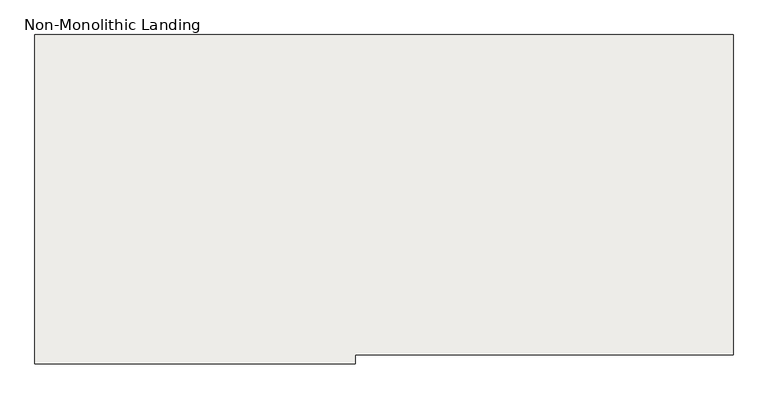
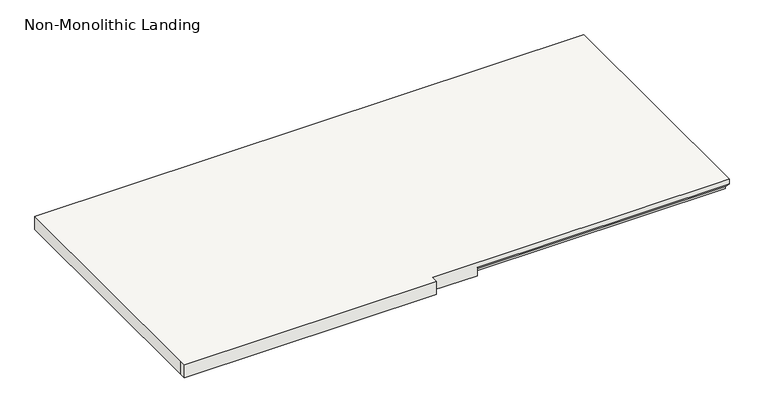
"""IFC4 building model written with IfcOpenShell, lengths in millimetres: slab geometry, Non-Monolithic Landing."""

from ifc_helpers import new_model, si_unit, origin, place, context, project, spatial, faceted_brep, source, transform, mapped, element, save


def non_monolithic_landing_8dc99a10(model_context):
    return source(origin(), model_context, "Body", "Brep", [
        faceted_brep([(-5380.4481169, -1269.3249317, 1919.8166667), (-5380.4481169, -1294.7249317, 1945.2166667), (-6294.8481169, -1294.7249317, 1945.2166667), (-6294.8481169, -1269.3249317, 1919.8166667), (-5380.4481169, -380.3249317, 1964.2666667), (-7372.0431792, -380.3249317, 1964.2666667), (-7372.0431792, -1294.7249317, 1964.2666667), (-7372.0431792, -1320.1249317, 1964.2666667), (-6457.6431792, -1320.1249317, 1964.2666667), (-6457.6431792, -1294.7249317, 1964.2666667), (-5380.4481169, -1294.7249317, 1964.2666667), (-6294.8481169, -1269.3249317, 1913.4666667), (-6294.8481169, -1294.7249317, 1913.4666667), (-6457.6431792, -1294.7249317, 1913.4666667), (-6457.6431792, -1320.1249317, 1913.4666667), (-7372.0431792, -1320.1249317, 1913.4666667), (-7372.0431792, -1294.7249317, 1913.4666667), (-7372.0431792, -380.3249317, 1913.4666667), (-5380.4481169, -380.3249317, 1913.4666667), (-5380.4481169, -1269.3249317, 1913.4666667)], [[[0, 1, 2, 3]], [[4, 5, 6, 7, 8, 9, 10]], [[11, 12, 13, 14, 15, 16, 17, 18, 19]], [[12, 11, 3, 2]], [[11, 19, 0, 3]], [[4, 10, 1, 0, 19, 18]], [[5, 4, 18, 17]], [[6, 5, 17, 16]], [[7, 6, 16, 15]], [[8, 7, 15, 14]], [[9, 8, 14, 13]], [[10, 9, 13, 12, 2, 1]]]),
    ])


if __name__ == "__main__":
    model = new_model("IFC4")
    model_context = context("Model", 3, world=origin())
    ifc_project = project(units=[si_unit("LENGTHUNIT", "METRE", prefix="MILLI")], contexts=[model_context])
    site = spatial("IfcSite", under=ifc_project)
    building = spatial("IfcBuilding", under=site)
    placement = place(None, origin())
    non_monolithic_landing_shape = non_monolithic_landing_8dc99a10(model_context)
    element("IfcSlab", 1, ObjectType="Non-Monolithic Landing", at=placement, inside=building, context=model_context, shape_type="MappedRepresentation", body=[
        mapped(non_monolithic_landing_shape, transform((0.0, 0.0, 0.0), x_axis=(1.0, 0.0, 0.0), y_axis=(0.0, 1.0, 0.0), z_axis=(0.0, 0.0, 1.0))),
    ])
    save(model, "model.ifc")
